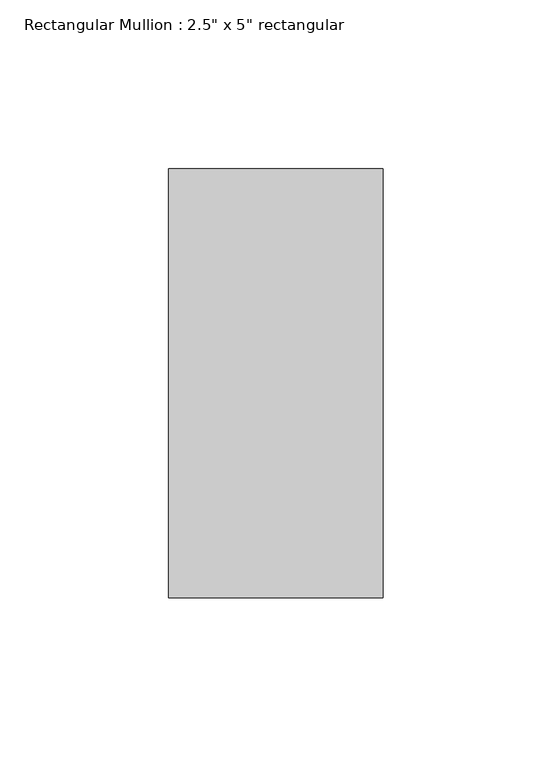
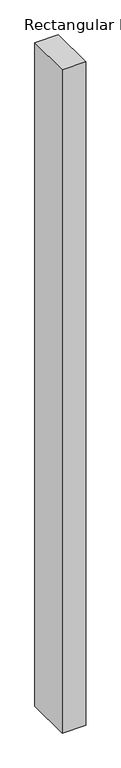
"""IFC4 building model written with IfcOpenShell, lengths in millimetres: member geometry."""

from ifc_helpers import new_model, si_unit, frame, origin, place, context, project, spatial, polyline, outline, extrude, source, transform, mapped, element, save


def member_33acc223(model_context):
    return source(origin(), model_context, "Body", "SweptSolid", [
        extrude(outline(polyline([(31.75, 63.5), (31.75, -63.5), (-31.75, -63.5), (-31.75, 63.5), (31.75, 63.5)])), frame((0.0, 0.0, -1889.1776273), z_axis=(0.0, 0.0, 1.0), x_axis=(1.0, 0.0, 0.0)), (0.0, 0.0, 1.0), 1889.1776273),
    ])


if __name__ == "__main__":
    model = new_model("IFC4")
    model_context = context("Model", 3, world=origin())
    ifc_project = project(units=[si_unit("LENGTHUNIT", "METRE", prefix="MILLI")], contexts=[model_context])
    site = spatial("IfcSite", under=ifc_project)
    building = spatial("IfcBuilding", under=site)
    placement = place(None, origin())
    member_shape = member_33acc223(model_context)
    element("IfcMember", 1, ObjectType="Rectangular Mullion : 2.5\" x 5\" rectangular", at=placement, inside=building, context=model_context, shape_type="MappedRepresentation", body=[
        mapped(member_shape, transform((0.0, 0.0, 0.0), x_axis=(1.0, 0.0, 0.0), y_axis=(0.0, 1.0, 0.0), z_axis=(0.0, 0.0, 1.0))),
    ])
    save(model, "model.ifc")

# Revit data of these elements
# Type "Rectangular Mullion : 2.5\" x 5\" rectangular"
#   built-in parameter 1007304 = 0.416667 (stored number, unit not read)
#   built-in parameter 1007301 = 0.104167 (stored number, unit not read)
#   built-in parameter 1007300 = 0.104167 (stored number, unit not read)
# Element 1 (IfcMember, "Rectangular Mullion : 2.5\" x 5\" rectangular")
#   Materials on its faces: "Aluminum"
# Materials
#   "Aluminum": class "Metal", colour RGB 247 247 247, transparency 0, Description = "Aluminum 6061", Cost = 0
